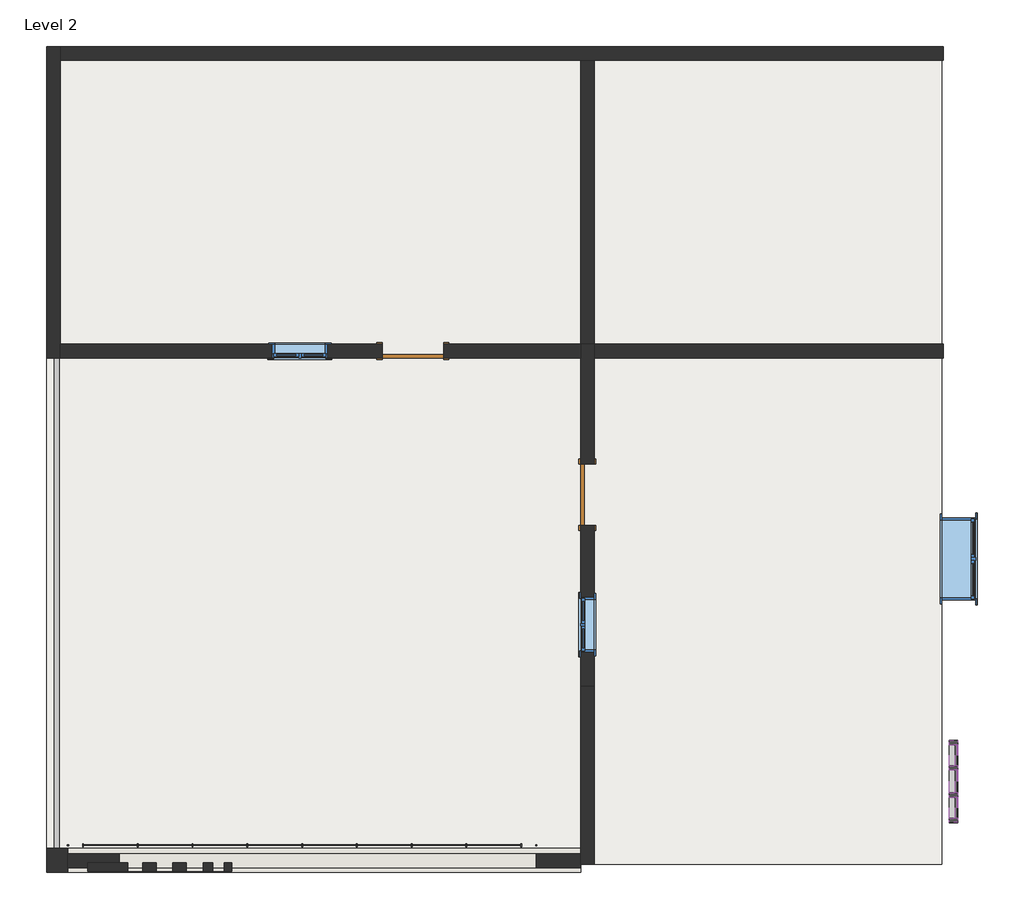
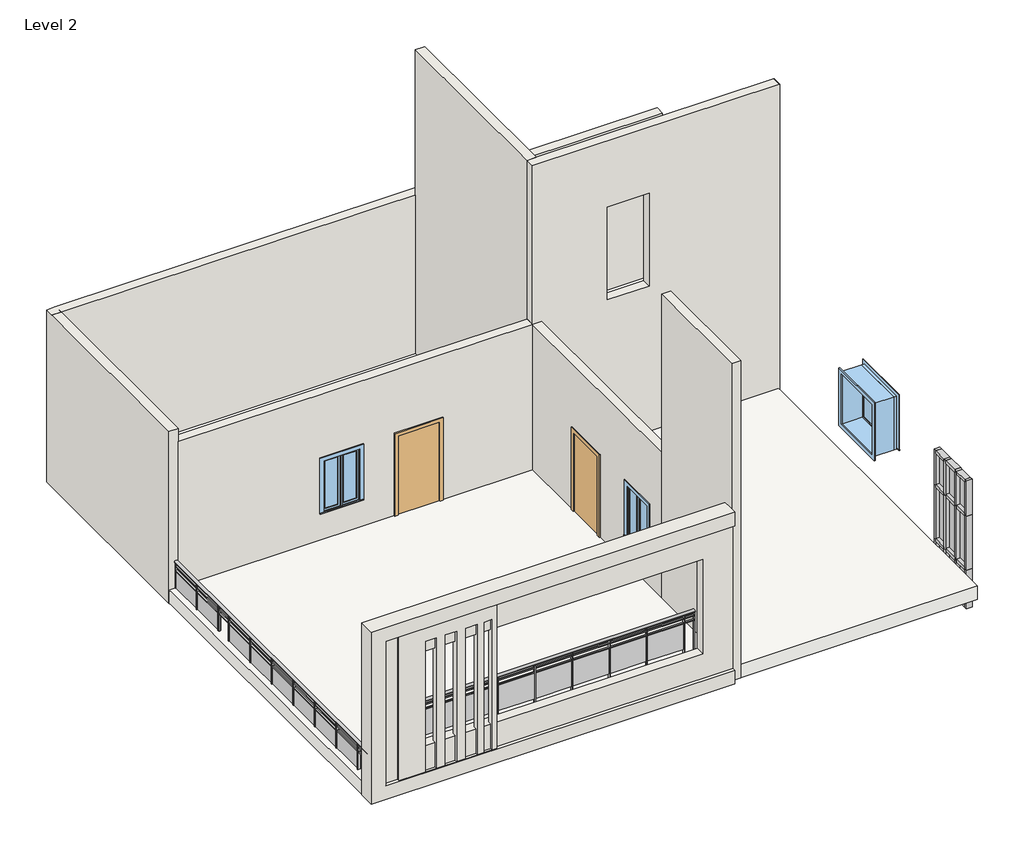
# One storey: 24 members, 10 walls, 9 plates, 3 windows, 2 doors, 2 railings, 1 roof.
"""IFC4 building model written with IfcOpenShell, lengths in millimetres."""

from ifc_helpers import new_model, si_unit, point, frame, origin, place, context, project, spatial, polyline, ellipse_curve, trimmed, outline, extrude, faceted_brep, transform, mapped, element, save
from ifc_brep_helpers import plane_surface, extruded_surface, advanced_brep
from components import door_54dd4da4, member_ff1b7d8f, member_5ad95953, member_5aeb4b7d, member_9850ab14, member_6e431393, member_26863f11, member_a1da5be3, member_58a4a87b, member_71eb4692, member_8b3492ed, system_panel_glazed_1557c927, system_panel_glazed_603fb926, system_panel_glazed_6328bcbd, system_panel_glazed_ea4b41a2, system_panel_glazed_510f06c2, system_panel_glazed_bd2ad356, walls_2_walls_2_aacfb59a, walls_3_walls_3_aaa7465c, window_bb17773d, window_25ed8443

model = new_model("IFC4")

# Units and contexts
model_context = context("Model", 3, world=origin())
ifc_project = project(units=[si_unit("LENGTHUNIT", "METRE", prefix="MILLI")], contexts=[model_context])

# Site, building, storey
site = spatial("IfcSite", under=ifc_project)
building = spatial("IfcBuilding", under=site)
storey = spatial("IfcBuildingStorey", under=building, Name="Level 2", Elevation=3657.6)

# Doors
placement = place(None, origin())
door_shape = door_54dd4da4(model_context)
element("IfcDoor", 1, ObjectType="Single-Flush : 36\" x 84\"", at=placement, inside=storey, context=model_context, shape_type="MappedRepresentation", body=[
    mapped(door_shape, transform((-6414.8745124, 6836.8609482, 3657.6), x_axis=(-1.0, 0.0, 0.0), y_axis=(0.0, -1.0, 0.0), z_axis=(0.0, 0.0, 1.0))),
])
element("IfcDoor", 2, ObjectType="Single-Flush : 36\" x 84\"", at=placement, inside=storey, context=model_context, shape_type="MappedRepresentation", body=[
    mapped(door_shape, transform((-3824.0745124, 4703.2609482, 3657.6), x_axis=(0.0, 1.0, 0.0), y_axis=(-1.0, 0.0, 0.0), z_axis=(0.0, 0.0, 1.0))),
])

# Members
member_shape = member_ff1b7d8f(model_context)
element("IfcMember", 3, ObjectType="Rectangular Mullion : 2.5\" x 5\" rectangular", at=placement, inside=storey, context=model_context, shape_type="MappedRepresentation", body=[
    mapped(member_shape, transform((1611.5254876, 617.0832725, 3022.9019988), x_axis=(0.0, 0.0, -1.0), y_axis=(-1.0, 0.0, 0.0), z_axis=(0.0, 1.0, 0.0))),
])
member_2_shape = member_5ad95953(model_context)
element("IfcMember", 4, ObjectType="Rectangular Mullion : 2.5\" x 5\" rectangular", at=placement, inside=storey, context=model_context, shape_type="MappedRepresentation", body=[
    mapped(member_2_shape, transform((1611.5254876, 210.6832725, 3022.9019988), x_axis=(0.0, 0.0, -1.0), y_axis=(-1.0, 0.0, 0.0), z_axis=(0.0, 1.0, 0.0))),
])
element("IfcMember", 5, ObjectType="Rectangular Mullion : 2.5\" x 5\" rectangular", at=placement, inside=storey, context=model_context, shape_type="MappedRepresentation", body=[
    mapped(member_2_shape, transform((1611.5254876, 991.7332725, 3022.9019988), x_axis=(0.0, 0.0, -1.0), y_axis=(-1.0, 0.0, 0.0), z_axis=(0.0, 1.0, 0.0))),
])
member_3_shape = member_5aeb4b7d(model_context)
element("IfcMember", 6, ObjectType="Rectangular Mullion : 2.5\" x 5\" rectangular", at=placement, inside=storey, context=model_context, shape_type="MappedRepresentation", body=[
    mapped(member_3_shape, transform((1611.5254876, 274.1832725, 3911.9019988), x_axis=(0.0, 0.0, 1.0), y_axis=(-1.0, 0.0, 0.0), z_axis=(0.0, -1.0, 0.0))),
])
element("IfcMember", 7, ObjectType="Rectangular Mullion : 2.5\" x 5\" rectangular", at=placement, inside=storey, context=model_context, shape_type="MappedRepresentation", body=[
    mapped(member_3_shape, transform((1611.5254876, 274.1832725, 5156.5019988), x_axis=(0.0, 0.0, 1.0), y_axis=(-1.0, 0.0, 0.0), z_axis=(0.0, -1.0, 0.0))),
])
member_4_shape = member_9850ab14(model_context)
element("IfcMember", 8, ObjectType="Rectangular Mullion : 2.5\" x 5\" rectangular", at=placement, inside=storey, context=model_context, shape_type="MappedRepresentation", body=[
    mapped(member_4_shape, transform((1611.5254876, -100.4667275, 3911.9019988), x_axis=(0.0, 0.0, 1.0), y_axis=(-1.0, 0.0, 0.0), z_axis=(0.0, -1.0, 0.0))),
])
element("IfcMember", 9, ObjectType="Rectangular Mullion : 2.5\" x 5\" rectangular", at=placement, inside=storey, context=model_context, shape_type="MappedRepresentation", body=[
    mapped(member_4_shape, transform((1611.5254876, 680.5832725, 3911.9019988), x_axis=(0.0, 0.0, 1.0), y_axis=(-1.0, 0.0, 0.0), z_axis=(0.0, -1.0, 0.0))),
])
element("IfcMember", 10, ObjectType="Rectangular Mullion : 2.5\" x 5\" rectangular", at=placement, inside=storey, context=model_context, shape_type="MappedRepresentation", body=[
    mapped(member_4_shape, transform((1611.5254876, -100.4667275, 5156.5019988), x_axis=(0.0, 0.0, 1.0), y_axis=(-1.0, 0.0, 0.0), z_axis=(0.0, -1.0, 0.0))),
])
element("IfcMember", 11, ObjectType="Rectangular Mullion : 2.5\" x 5\" rectangular", at=placement, inside=storey, context=model_context, shape_type="MappedRepresentation", body=[
    mapped(member_4_shape, transform((1611.5254876, 680.5832725, 5156.5019988), x_axis=(0.0, 0.0, 1.0), y_axis=(-1.0, 0.0, 0.0), z_axis=(0.0, -1.0, 0.0))),
])
element("IfcMember", 12, ObjectType="Rectangular Mullion : 2.5\" x 5\" rectangular", at=placement, inside=storey, context=model_context, shape_type="MappedRepresentation", body=[
    mapped(member_2_shape, transform((1611.5254876, 680.5832725, 5969.3019988), x_axis=(0.0, 0.0, 1.0), y_axis=(-1.0, 0.0, 0.0), z_axis=(0.0, -1.0, 0.0))),
])
element("IfcMember", 13, ObjectType="Rectangular Mullion : 2.5\" x 5\" rectangular", at=placement, inside=storey, context=model_context, shape_type="MappedRepresentation", body=[
    mapped(member_2_shape, transform((1611.5254876, -100.4667275, 5969.3019988), x_axis=(0.0, 0.0, 1.0), y_axis=(-1.0, 0.0, 0.0), z_axis=(0.0, -1.0, 0.0))),
])
element("IfcMember", 14, ObjectType="Rectangular Mullion : 2.5\" x 5\" rectangular", at=placement, inside=storey, context=model_context, shape_type="MappedRepresentation", body=[
    mapped(member_shape, transform((1611.5254876, 274.1832725, 5969.3019988), x_axis=(0.0, 0.0, 1.0), y_axis=(-1.0, 0.0, 0.0), z_axis=(0.0, -1.0, 0.0))),
])
member_5_shape = member_6e431393(model_context)
element("IfcMember", 15, ObjectType="Rectangular Mullion : 2.5\" x 5\" rectangular", at=placement, inside=storey, context=model_context, shape_type="MappedRepresentation", body=[
    mapped(member_5_shape, transform((1611.5254876, 648.8332725, 3022.9019988), x_axis=(0.0, -1.0, 0.0), y_axis=(-1.0, 0.0, 0.0), z_axis=(0.0, 0.0, -1.0))),
])
element("IfcMember", 16, ObjectType="Rectangular Mullion : 2.5\" x 5\" rectangular", at=placement, inside=storey, context=model_context, shape_type="MappedRepresentation", body=[
    mapped(member_5_shape, transform((1611.5254876, 242.4332725, 3022.9019988), x_axis=(0.0, -1.0, 0.0), y_axis=(-1.0, 0.0, 0.0), z_axis=(0.0, 0.0, -1.0))),
])
member_6_shape = member_26863f11(model_context)
element("IfcMember", 17, ObjectType="Rectangular Mullion : 2.5\" x 5\" rectangular", at=placement, inside=storey, context=model_context, shape_type="MappedRepresentation", body=[
    mapped(member_6_shape, transform((1611.5254876, -163.9667275, 3022.9019988), x_axis=(0.0, -1.0, 0.0), y_axis=(-1.0, 0.0, 0.0), z_axis=(0.0, 0.0, -1.0))),
])
element("IfcMember", 18, ObjectType="Rectangular Mullion : 2.5\" x 5\" rectangular", at=placement, inside=storey, context=model_context, shape_type="MappedRepresentation", body=[
    mapped(member_6_shape, transform((1611.5254876, 1055.2332725, 3911.9019988), x_axis=(0.0, 1.0, 0.0), y_axis=(-1.0, 0.0, 0.0), z_axis=(0.0, 0.0, 1.0))),
])
member_7_shape = member_a1da5be3(model_context)
element("IfcMember", 19, ObjectType="Rectangular Mullion : 2.5\" x 5\" rectangular", at=placement, inside=storey, context=model_context, shape_type="MappedRepresentation", body=[
    mapped(member_7_shape, transform((1611.5254876, 648.8332725, 3911.9019988), x_axis=(0.0, -1.0, 0.0), y_axis=(-1.0, 0.0, 0.0), z_axis=(0.0, 0.0, -1.0))),
])
element("IfcMember", 20, ObjectType="Rectangular Mullion : 2.5\" x 5\" rectangular", at=placement, inside=storey, context=model_context, shape_type="MappedRepresentation", body=[
    mapped(member_7_shape, transform((1611.5254876, 242.4332725, 3911.9019988), x_axis=(0.0, -1.0, 0.0), y_axis=(-1.0, 0.0, 0.0), z_axis=(0.0, 0.0, -1.0))),
])
member_8_shape = member_58a4a87b(model_context)
element("IfcMember", 21, ObjectType="Rectangular Mullion : 2.5\" x 5\" rectangular", at=placement, inside=storey, context=model_context, shape_type="MappedRepresentation", body=[
    mapped(member_8_shape, transform((1611.5254876, 648.8332725, 5156.5019988), x_axis=(0.0, -1.0, 0.0), y_axis=(-1.0, 0.0, 0.0), z_axis=(0.0, 0.0, -1.0))),
])
element("IfcMember", 22, ObjectType="Rectangular Mullion : 2.5\" x 5\" rectangular", at=placement, inside=storey, context=model_context, shape_type="MappedRepresentation", body=[
    mapped(member_8_shape, transform((1611.5254876, 242.4332725, 5156.5019988), x_axis=(0.0, -1.0, 0.0), y_axis=(-1.0, 0.0, 0.0), z_axis=(0.0, 0.0, -1.0))),
])
member_9_shape = member_71eb4692(model_context)
element("IfcMember", 23, ObjectType="Rectangular Mullion : 2.5\" x 5\" rectangular", at=placement, inside=storey, context=model_context, shape_type="MappedRepresentation", body=[
    mapped(member_9_shape, transform((1611.5254876, -163.9667275, 3911.9019988), x_axis=(0.0, -1.0, 0.0), y_axis=(-1.0, 0.0, 0.0), z_axis=(0.0, 0.0, -1.0))),
])
member_10_shape = member_8b3492ed(model_context)
element("IfcMember", 24, ObjectType="Rectangular Mullion : 2.5\" x 5\" rectangular", at=placement, inside=storey, context=model_context, shape_type="MappedRepresentation", body=[
    mapped(member_10_shape, transform((1611.5254876, -163.9667275, 5156.5019988), x_axis=(0.0, -1.0, 0.0), y_axis=(-1.0, 0.0, 0.0), z_axis=(0.0, 0.0, -1.0))),
])
element("IfcMember", 25, ObjectType="Rectangular Mullion : 2.5\" x 5\" rectangular", at=placement, inside=storey, context=model_context, shape_type="MappedRepresentation", body=[
    mapped(member_9_shape, transform((1611.5254876, 1055.2332725, 5156.5019988), x_axis=(0.0, 1.0, 0.0), y_axis=(-1.0, 0.0, 0.0), z_axis=(0.0, 0.0, 1.0))),
])
element("IfcMember", 26, ObjectType="Rectangular Mullion : 2.5\" x 5\" rectangular", at=placement, inside=storey, context=model_context, shape_type="MappedRepresentation", body=[
    mapped(member_10_shape, transform((1611.5254876, 1055.2332725, 5969.3019988), x_axis=(0.0, 1.0, 0.0), y_axis=(-1.0, 0.0, 0.0), z_axis=(0.0, 0.0, 1.0))),
])

# Plates
system_panel_glazed_shape = system_panel_glazed_1557c927(model_context)
element("IfcPlate", 27, ObjectType="System Panel : Glazed", at=placement, inside=storey, context=model_context, shape_type="MappedRepresentation", body=[
    mapped(system_panel_glazed_shape, transform((1611.5254876, 836.1582725, 3086.4019988), x_axis=(0.0, -1.0, 0.0), y_axis=(1.0, 0.0, 0.0), z_axis=(0.0, 0.0, 1.0))),
])
element("IfcPlate", 28, ObjectType="System Panel : Glazed", at=placement, inside=storey, context=model_context, shape_type="MappedRepresentation", body=[
    mapped(system_panel_glazed_shape, transform((1611.5254876, 55.1082725, 3086.4019988), x_axis=(0.0, -1.0, 0.0), y_axis=(1.0, 0.0, 0.0), z_axis=(0.0, 0.0, 1.0))),
])
system_panel_glazed_2_shape = system_panel_glazed_603fb926(model_context)
element("IfcPlate", 29, ObjectType="System Panel : Glazed", at=placement, inside=storey, context=model_context, shape_type="MappedRepresentation", body=[
    mapped(system_panel_glazed_2_shape, transform((1611.5254876, 445.6332725, 3086.4019988), x_axis=(0.0, -1.0, 0.0), y_axis=(1.0, 0.0, 0.0), z_axis=(0.0, 0.0, 1.0))),
])
system_panel_glazed_3_shape = system_panel_glazed_6328bcbd(model_context)
element("IfcPlate", 30, ObjectType="System Panel : Glazed", at=placement, inside=storey, context=model_context, shape_type="MappedRepresentation", body=[
    mapped(system_panel_glazed_3_shape, transform((1611.5254876, 836.1582725, 5188.2519988), x_axis=(0.0, -1.0, 0.0), y_axis=(1.0, 0.0, 0.0), z_axis=(0.0, 0.0, 1.0))),
])
element("IfcPlate", 31, ObjectType="System Panel : Glazed", at=placement, inside=storey, context=model_context, shape_type="MappedRepresentation", body=[
    mapped(system_panel_glazed_3_shape, transform((1611.5254876, 55.1082725, 5188.2519988), x_axis=(0.0, -1.0, 0.0), y_axis=(1.0, 0.0, 0.0), z_axis=(0.0, 0.0, 1.0))),
])
system_panel_glazed_4_shape = system_panel_glazed_ea4b41a2(model_context)
element("IfcPlate", 32, ObjectType="System Panel : Glazed", at=placement, inside=storey, context=model_context, shape_type="MappedRepresentation", body=[
    mapped(system_panel_glazed_4_shape, transform((1611.5254876, 445.6332725, 5188.2519988), x_axis=(0.0, -1.0, 0.0), y_axis=(1.0, 0.0, 0.0), z_axis=(0.0, 0.0, 1.0))),
])
system_panel_glazed_5_shape = system_panel_glazed_510f06c2(model_context)
element("IfcPlate", 33, ObjectType="System Panel : Glazed", at=placement, inside=storey, context=model_context, shape_type="MappedRepresentation", body=[
    mapped(system_panel_glazed_5_shape, transform((1611.5254876, 836.1582725, 3943.6519988), x_axis=(0.0, -1.0, 0.0), y_axis=(1.0, 0.0, 0.0), z_axis=(0.0, 0.0, 1.0))),
])
element("IfcPlate", 34, ObjectType="System Panel : Glazed", at=placement, inside=storey, context=model_context, shape_type="MappedRepresentation", body=[
    mapped(system_panel_glazed_5_shape, transform((1611.5254876, 55.1082725, 3943.6519988), x_axis=(0.0, -1.0, 0.0), y_axis=(1.0, 0.0, 0.0), z_axis=(0.0, 0.0, 1.0))),
])
system_panel_glazed_6_shape = system_panel_glazed_bd2ad356(model_context)
element("IfcPlate", 35, ObjectType="System Panel : Glazed", at=placement, inside=storey, context=model_context, shape_type="MappedRepresentation", body=[
    mapped(system_panel_glazed_6_shape, transform((1611.5254876, 445.6332725, 3943.6519988), x_axis=(0.0, -1.0, 0.0), y_axis=(1.0, 0.0, 0.0), z_axis=(0.0, 0.0, 1.0))),
])

# Railings
element("IfcRailing", 36, ObjectType="Glass Panel - Bottom Fill", at=placement, inside=storey, context=model_context, shape_type="SolidModel", body=[
    advanced_brep(
    [(-11535.2764802, -464.1328007, 5334.0), (-11535.2764802, -540.3328007, 5334.0), (-4580.8162469, -464.1328007, 5334.0), (-4580.8162469, -540.3328007, 5334.0)],
    [
        (0, 1, ellipse_curve(frame((-11535.2764802, -502.2328007, 5334.0), z_axis=(-1.0, 0.0, 0.0), x_axis=(0.0, -1.0, 0.0)), 38.1, 28.575)),
        (1, 0, ellipse_curve(frame((-11535.2764802, -502.2328007, 5334.0), z_axis=(-1.0, 0.0, 0.0), x_axis=(0.0, -1.0, 0.0)), 38.1, 28.575)),
        (2, 3, ellipse_curve(frame((-4580.8162469, -502.2328007, 5334.0), z_axis=(1.0, 0.0, 0.0), x_axis=(0.0, -1.0, 0.0)), 38.1, 28.575)),
        (3, 2, ellipse_curve(frame((-4580.8162469, -502.2328007, 5334.0), z_axis=(1.0, 0.0, 0.0), x_axis=(0.0, -1.0, 0.0)), 38.1, 28.575)),
        (0, 2),
        (3, 1),
    ],
    [
        plane_surface(frame((-11535.2764802, -502.2328007, 5334.0), z_axis=(-1.0, 0.0, 0.0), x_axis=(0.0, 1.0, 0.0))),
        plane_surface(frame((-4580.8162469, -502.2328007, 5334.0), z_axis=(1.0, 0.0, 0.0), x_axis=(0.0, 1.0, 0.0))),
        extruded_surface(trimmed(ellipse_curve(frame((-4580.8162469, -502.2328007, 5334.0), z_axis=(-1.0, 0.0, 0.0), x_axis=(0.0, -1.0, 0.0)), 38.1, 28.575), [point((-4580.8162469, -464.1328007, 5334.0))], [point((-4580.8162469, -540.3328007, 5334.0))], True, "CARTESIAN"), (-6954.4602333, 0.0, 0.0), 6954.4602333),
        extruded_surface(trimmed(ellipse_curve(frame((-4580.8162469, -502.2328007, 5334.0), z_axis=(-1.0, 0.0, 0.0), x_axis=(0.0, -1.0, 0.0)), 38.1, 28.575), [point((-4580.8162469, -540.3328007, 5334.0))], [point((-4580.8162469, -464.1328007, 5334.0))], True, "CARTESIAN"), (-6954.4602333, 0.0, 0.0), 6954.4602333),
    ],
    [
        (0, [[1, 2]]),
        (1, [[3, 4]]),
        (2, [[-1, 5, -4, 6]]),
        (3, [[-2, -6, -3, -5]]),
    ],
),
    extrude(outline(polyline([(-11535.2764802, -514.9328007), (-11535.2764802, -489.5328007), (-4580.8162469, -489.5328007), (-4580.8162469, -514.9328007), (-11535.2764802, -514.9328007)])), frame((0.0, 0.0, 5219.7), z_axis=(0.0, 0.0, 1.0), x_axis=(1.0, 0.0, 0.0)), (0.0, 0.0, 1.0), 25.4),
    extrude(outline(polyline([(-11535.2764802, -514.9328007), (-11535.2764802, -489.5328007), (-4580.8162469, -489.5328007), (-4580.8162469, -514.9328007), (-11535.2764802, -514.9328007)])), frame((0.0, 0.0, 5118.1), z_axis=(0.0, 0.0, 1.0), x_axis=(1.0, 0.0, 0.0)), (0.0, 0.0, 1.0), 25.4),
    extrude(outline(polyline([(-4813.1963636, -527.6328007), (-4813.1963636, -476.8328007), (-4800.4963636, -476.8328007), (-4800.4963636, -527.6328007), (-4813.1963636, -527.6328007)])), frame((0.0, 0.0, 4419.6), z_axis=(0.0, 0.0, 1.0), x_axis=(1.0, 0.0, 0.0)), (0.0, 0.0, 1.0), 885.6788223),
    extrude(outline(polyline([(-5619.6463636, -495.6976436), (-4806.8463636, -495.6976436), (-4806.8463636, -502.0476436), (-5619.6463636, -502.0476436), (-5619.6463636, -495.6976436)])), frame((0.0, 0.0, 4521.2), z_axis=(0.0, 0.0, 1.0), x_axis=(1.0, 0.0, 0.0)), (0.0, 0.0, 1.0), 596.9),
    extrude(outline(polyline([(-5625.9963636, -527.6328007), (-5625.9963636, -476.8328007), (-5613.2963636, -476.8328007), (-5613.2963636, -527.6328007), (-5625.9963636, -527.6328007)])), frame((0.0, 0.0, 4419.6), z_axis=(0.0, 0.0, 1.0), x_axis=(1.0, 0.0, 0.0)), (0.0, 0.0, 1.0), 885.6788223),
    extrude(outline(polyline([(-6432.4463636, -495.6976436), (-5619.6463636, -495.6976436), (-5619.6463636, -502.0476436), (-6432.4463636, -502.0476436), (-6432.4463636, -495.6976436)])), frame((0.0, 0.0, 4521.2), z_axis=(0.0, 0.0, 1.0), x_axis=(1.0, 0.0, 0.0)), (0.0, 0.0, 1.0), 596.9),
    extrude(outline(polyline([(-6438.7963636, -527.6328007), (-6438.7963636, -476.8328007), (-6426.0963636, -476.8328007), (-6426.0963636, -527.6328007), (-6438.7963636, -527.6328007)])), frame((0.0, 0.0, 4419.6), z_axis=(0.0, 0.0, 1.0), x_axis=(1.0, 0.0, 0.0)), (0.0, 0.0, 1.0), 885.6788223),
    extrude(outline(polyline([(-7245.2463636, -495.6976436), (-6432.4463636, -495.6976436), (-6432.4463636, -502.0476436), (-7245.2463636, -502.0476436), (-7245.2463636, -495.6976436)])), frame((0.0, 0.0, 4521.2), z_axis=(0.0, 0.0, 1.0), x_axis=(1.0, 0.0, 0.0)), (0.0, 0.0, 1.0), 596.9),
    extrude(outline(polyline([(-7251.5963636, -527.6328007), (-7251.5963636, -476.8328007), (-7238.8963636, -476.8328007), (-7238.8963636, -527.6328007), (-7251.5963636, -527.6328007)])), frame((0.0, 0.0, 4419.6), z_axis=(0.0, 0.0, 1.0), x_axis=(1.0, 0.0, 0.0)), (0.0, 0.0, 1.0), 885.6788223),
    extrude(outline(polyline([(-8058.0463636, -495.6976436), (-7245.2463636, -495.6976436), (-7245.2463636, -502.0476436), (-8058.0463636, -502.0476436), (-8058.0463636, -495.6976436)])), frame((0.0, 0.0, 4521.2), z_axis=(0.0, 0.0, 1.0), x_axis=(1.0, 0.0, 0.0)), (0.0, 0.0, 1.0), 596.9),
    extrude(outline(polyline([(-8064.3963636, -527.6328007), (-8064.3963636, -476.8328007), (-8051.6963636, -476.8328007), (-8051.6963636, -527.6328007), (-8064.3963636, -527.6328007)])), frame((0.0, 0.0, 4419.6), z_axis=(0.0, 0.0, 1.0), x_axis=(1.0, 0.0, 0.0)), (0.0, 0.0, 1.0), 885.6788223),
    extrude(outline(polyline([(-8870.8463636, -495.6976436), (-8058.0463636, -495.6976436), (-8058.0463636, -502.0476436), (-8870.8463636, -502.0476436), (-8870.8463636, -495.6976436)])), frame((0.0, 0.0, 4521.2), z_axis=(0.0, 0.0, 1.0), x_axis=(1.0, 0.0, 0.0)), (0.0, 0.0, 1.0), 596.9),
    extrude(outline(polyline([(-8877.1963636, -527.6328007), (-8877.1963636, -476.8328007), (-8864.4963636, -476.8328007), (-8864.4963636, -527.6328007), (-8877.1963636, -527.6328007)])), frame((0.0, 0.0, 4419.6), z_axis=(0.0, 0.0, 1.0), x_axis=(1.0, 0.0, 0.0)), (0.0, 0.0, 1.0), 885.6788223),
    extrude(outline(polyline([(-9683.6463636, -495.6976436), (-8870.8463636, -495.6976436), (-8870.8463636, -502.0476436), (-9683.6463636, -502.0476436), (-9683.6463636, -495.6976436)])), frame((0.0, 0.0, 4521.2), z_axis=(0.0, 0.0, 1.0), x_axis=(1.0, 0.0, 0.0)), (0.0, 0.0, 1.0), 596.9),
    extrude(outline(polyline([(-9689.9963636, -527.6328007), (-9689.9963636, -476.8328007), (-9677.2963636, -476.8328007), (-9677.2963636, -527.6328007), (-9689.9963636, -527.6328007)])), frame((0.0, 0.0, 4419.6), z_axis=(0.0, 0.0, 1.0), x_axis=(1.0, 0.0, 0.0)), (0.0, 0.0, 1.0), 885.6788223),
    extrude(outline(polyline([(-10496.4463636, -495.6976436), (-9683.6463636, -495.6976436), (-9683.6463636, -502.0476436), (-10496.4463636, -502.0476436), (-10496.4463636, -495.6976436)])), frame((0.0, 0.0, 4521.2), z_axis=(0.0, 0.0, 1.0), x_axis=(1.0, 0.0, 0.0)), (0.0, 0.0, 1.0), 596.9),
    extrude(outline(polyline([(-10502.7963636, -527.6328007), (-10502.7963636, -476.8328007), (-10490.0963636, -476.8328007), (-10490.0963636, -527.6328007), (-10502.7963636, -527.6328007)])), frame((0.0, 0.0, 4419.6), z_axis=(0.0, 0.0, 1.0), x_axis=(1.0, 0.0, 0.0)), (0.0, 0.0, 1.0), 885.6788223),
    extrude(outline(polyline([(-11309.2463636, -495.6976436), (-10496.4463636, -495.6976436), (-10496.4463636, -502.0476436), (-11309.2463636, -502.0476436), (-11309.2463636, -495.6976436)])), frame((0.0, 0.0, 4521.2), z_axis=(0.0, 0.0, 1.0), x_axis=(1.0, 0.0, 0.0)), (0.0, 0.0, 1.0), 596.9),
    extrude(outline(polyline([(-11315.5963636, -527.6328007), (-11315.5963636, -476.8328007), (-11302.8963636, -476.8328007), (-11302.8963636, -527.6328007), (-11315.5963636, -527.6328007)])), frame((0.0, 0.0, 4419.6), z_axis=(0.0, 0.0, 1.0), x_axis=(1.0, 0.0, 0.0)), (0.0, 0.0, 1.0), 885.6788223),
    extrude(outline(polyline([(-4593.5162469, -511.7578007), (-4593.5162469, -492.7078007), (-4574.4662469, -492.7078007), (-4574.4662469, -511.7578007), (-4593.5162469, -511.7578007)])), frame((0.0, 0.0, 4419.6), z_axis=(0.0, 0.0, 1.0), x_axis=(1.0, 0.0, 0.0)), (0.0, 0.0, 1.0), 885.6788223),
    extrude(outline(polyline([(-11541.6264802, -511.7578007), (-11541.6264802, -492.7078007), (-11522.5764802, -492.7078007), (-11522.5764802, -511.7578007), (-11541.6264802, -511.7578007)])), frame((0.0, 0.0, 4419.6), z_axis=(0.0, 0.0, 1.0), x_axis=(1.0, 0.0, 0.0)), (0.0, 0.0, 1.0), 885.6788223),
])
element("IfcRailing", 37, ObjectType="Glass Panel - Bottom Fill", at=placement, inside=storey, context=model_context, shape_type="SolidModel", body=[
    advanced_brep(
    [(-11736.1745124, -545.7345899, 4572.0), (-11659.9745124, -545.7345899, 4572.0), (-11736.1745124, 6735.2609482, 4572.0), (-11659.9745124, 6735.2609482, 4572.0)],
    [
        (0, 1, ellipse_curve(frame((-11698.0745124, -545.7345899, 4572.0), z_axis=(0.0, -1.0, 0.0), x_axis=(1.0, 0.0, 0.0)), 38.1, 28.575)),
        (1, 0, ellipse_curve(frame((-11698.0745124, -545.7345899, 4572.0), z_axis=(0.0, -1.0, 0.0), x_axis=(1.0, 0.0, 0.0)), 38.1, 28.575)),
        (2, 3, ellipse_curve(frame((-11698.0745124, 6735.2609482, 4572.0), z_axis=(0.0, 1.0, 0.0), x_axis=(1.0, 0.0, 0.0)), 38.1, 28.575)),
        (3, 2, ellipse_curve(frame((-11698.0745124, 6735.2609482, 4572.0), z_axis=(0.0, 1.0, 0.0), x_axis=(1.0, 0.0, 0.0)), 38.1, 28.575)),
        (0, 2),
        (3, 1),
    ],
    [
        plane_surface(frame((-11698.0745124, -545.7345899, 4572.0), z_axis=(0.0, -1.0, 0.0), x_axis=(0.0, 0.0, 1.0))),
        plane_surface(frame((-11698.0745124, 6735.2609482, 4572.0), z_axis=(0.0, 1.0, 0.0), x_axis=(0.0, 0.0, 1.0))),
        extruded_surface(trimmed(ellipse_curve(frame((-11698.0745124, 6735.2609482, 4572.0), z_axis=(0.0, -1.0, 0.0), x_axis=(1.0, 0.0, 0.0)), 38.1, 28.575), [point((-11736.1745124, 6735.2609482, 4572.0))], [point((-11659.9745124, 6735.2609482, 4572.0))], True, "CARTESIAN"), (0.0, -7280.9955381, 0.0), 7280.9955381),
        extruded_surface(trimmed(ellipse_curve(frame((-11698.0745124, 6735.2609482, 4572.0), z_axis=(0.0, -1.0, 0.0), x_axis=(1.0, 0.0, 0.0)), 38.1, 28.575), [point((-11659.9745124, 6735.2609482, 4572.0))], [point((-11736.1745124, 6735.2609482, 4572.0))], True, "CARTESIAN"), (0.0, -7280.9955381, 0.0), 7280.9955381),
    ],
    [
        (0, [[1, 2]]),
        (1, [[3, 4]]),
        (2, [[-1, 5, -4, 6]]),
        (3, [[-2, -6, -3, -5]]),
    ],
),
    extrude(outline(polyline([(-11685.3745124, -545.7345899), (-11710.7745124, -545.7345899), (-11710.7745124, 6735.2609482), (-11685.3745124, 6735.2609482), (-11685.3745124, -545.7345899)])), frame((0.0, 0.0, 4457.7), z_axis=(0.0, 0.0, 1.0), x_axis=(1.0, 0.0, 0.0)), (0.0, 0.0, 1.0), 25.4),
    extrude(outline(polyline([(-11685.3745124, -545.7345899), (-11710.7745124, -545.7345899), (-11710.7745124, 6735.2609482), (-11685.3745124, 6735.2609482), (-11685.3745124, -545.7345899)])), frame((0.0, 0.0, 4356.1), z_axis=(0.0, 0.0, 1.0), x_axis=(1.0, 0.0, 0.0)), (0.0, 0.0, 1.0), 25.4),
    extrude(outline(polyline([(-11672.6745124, 6720.6131791), (-11723.4745124, 6720.6131791), (-11723.4745124, 6733.3131791), (-11672.6745124, 6733.3131791), (-11672.6745124, 6720.6131791)])), frame((0.0, 0.0, 3657.6), z_axis=(0.0, 0.0, 1.0), x_axis=(1.0, 0.0, 0.0)), (0.0, 0.0, 1.0), 885.6788223),
    extrude(outline(polyline([(-11704.6096694, 5914.1631791), (-11704.6096694, 6726.9631791), (-11698.2596694, 6726.9631791), (-11698.2596694, 5914.1631791), (-11704.6096694, 5914.1631791)])), frame((0.0, 0.0, 3759.2), z_axis=(0.0, 0.0, 1.0), x_axis=(1.0, 0.0, 0.0)), (0.0, 0.0, 1.0), 596.9),
    extrude(outline(polyline([(-11672.6745124, 5907.8131791), (-11723.4745124, 5907.8131791), (-11723.4745124, 5920.5131791), (-11672.6745124, 5920.5131791), (-11672.6745124, 5907.8131791)])), frame((0.0, 0.0, 3657.6), z_axis=(0.0, 0.0, 1.0), x_axis=(1.0, 0.0, 0.0)), (0.0, 0.0, 1.0), 885.6788223),
    extrude(outline(polyline([(-11704.6096694, 5101.3631791), (-11704.6096694, 5914.1631791), (-11698.2596694, 5914.1631791), (-11698.2596694, 5101.3631791), (-11704.6096694, 5101.3631791)])), frame((0.0, 0.0, 3759.2), z_axis=(0.0, 0.0, 1.0), x_axis=(1.0, 0.0, 0.0)), (0.0, 0.0, 1.0), 596.9),
    extrude(outline(polyline([(-11672.6745124, 5095.0131791), (-11723.4745124, 5095.0131791), (-11723.4745124, 5107.7131791), (-11672.6745124, 5107.7131791), (-11672.6745124, 5095.0131791)])), frame((0.0, 0.0, 3657.6), z_axis=(0.0, 0.0, 1.0), x_axis=(1.0, 0.0, 0.0)), (0.0, 0.0, 1.0), 885.6788223),
    extrude(outline(polyline([(-11672.6745124, 4705.7154101), (-11723.4745124, 4705.7154101), (-11723.4745124, 4718.4154101), (-11672.6745124, 4718.4154101), (-11672.6745124, 4705.7154101)])), frame((0.0, 0.0, 3657.6), z_axis=(0.0, 0.0, 1.0), x_axis=(1.0, 0.0, 0.0)), (0.0, 0.0, 1.0), 885.6788223),
    extrude(outline(polyline([(-11704.6096694, 3899.2654101), (-11704.6096694, 4712.0654101), (-11698.2596694, 4712.0654101), (-11698.2596694, 3899.2654101), (-11704.6096694, 3899.2654101)])), frame((0.0, 0.0, 3759.2), z_axis=(0.0, 0.0, 1.0), x_axis=(1.0, 0.0, 0.0)), (0.0, 0.0, 1.0), 596.9),
    extrude(outline(polyline([(-11672.6745124, 3892.9154101), (-11723.4745124, 3892.9154101), (-11723.4745124, 3905.6154101), (-11672.6745124, 3905.6154101), (-11672.6745124, 3892.9154101)])), frame((0.0, 0.0, 3657.6), z_axis=(0.0, 0.0, 1.0), x_axis=(1.0, 0.0, 0.0)), (0.0, 0.0, 1.0), 885.6788223),
    extrude(outline(polyline([(-11704.6096694, 3086.4654101), (-11704.6096694, 3899.2654101), (-11698.2596694, 3899.2654101), (-11698.2596694, 3086.4654101), (-11704.6096694, 3086.4654101)])), frame((0.0, 0.0, 3759.2), z_axis=(0.0, 0.0, 1.0), x_axis=(1.0, 0.0, 0.0)), (0.0, 0.0, 1.0), 596.9),
    extrude(outline(polyline([(-11672.6745124, 3080.1154101), (-11723.4745124, 3080.1154101), (-11723.4745124, 3092.8154101), (-11672.6745124, 3092.8154101), (-11672.6745124, 3080.1154101)])), frame((0.0, 0.0, 3657.6), z_axis=(0.0, 0.0, 1.0), x_axis=(1.0, 0.0, 0.0)), (0.0, 0.0, 1.0), 885.6788223),
    extrude(outline(polyline([(-11704.6096694, 2273.6654101), (-11704.6096694, 3086.4654101), (-11698.2596694, 3086.4654101), (-11698.2596694, 2273.6654101), (-11704.6096694, 2273.6654101)])), frame((0.0, 0.0, 3759.2), z_axis=(0.0, 0.0, 1.0), x_axis=(1.0, 0.0, 0.0)), (0.0, 0.0, 1.0), 596.9),
    extrude(outline(polyline([(-11672.6745124, 2267.3154101), (-11723.4745124, 2267.3154101), (-11723.4745124, 2280.0154101), (-11672.6745124, 2280.0154101), (-11672.6745124, 2267.3154101)])), frame((0.0, 0.0, 3657.6), z_axis=(0.0, 0.0, 1.0), x_axis=(1.0, 0.0, 0.0)), (0.0, 0.0, 1.0), 885.6788223),
    extrude(outline(polyline([(-11704.6096694, 1460.8654101), (-11704.6096694, 2273.6654101), (-11698.2596694, 2273.6654101), (-11698.2596694, 1460.8654101), (-11704.6096694, 1460.8654101)])), frame((0.0, 0.0, 3759.2), z_axis=(0.0, 0.0, 1.0), x_axis=(1.0, 0.0, 0.0)), (0.0, 0.0, 1.0), 596.9),
    extrude(outline(polyline([(-11672.6745124, 1454.5154101), (-11723.4745124, 1454.5154101), (-11723.4745124, 1467.2154101), (-11672.6745124, 1467.2154101), (-11672.6745124, 1454.5154101)])), frame((0.0, 0.0, 3657.6), z_axis=(0.0, 0.0, 1.0), x_axis=(1.0, 0.0, 0.0)), (0.0, 0.0, 1.0), 885.6788223),
    extrude(outline(polyline([(-11704.6096694, 648.0654101), (-11704.6096694, 1460.8654101), (-11698.2596694, 1460.8654101), (-11698.2596694, 648.0654101), (-11704.6096694, 648.0654101)])), frame((0.0, 0.0, 3759.2), z_axis=(0.0, 0.0, 1.0), x_axis=(1.0, 0.0, 0.0)), (0.0, 0.0, 1.0), 596.9),
    extrude(outline(polyline([(-11672.6745124, 641.7154101), (-11723.4745124, 641.7154101), (-11723.4745124, 654.4154101), (-11672.6745124, 654.4154101), (-11672.6745124, 641.7154101)])), frame((0.0, 0.0, 3657.6), z_axis=(0.0, 0.0, 1.0), x_axis=(1.0, 0.0, 0.0)), (0.0, 0.0, 1.0), 885.6788223),
    extrude(outline(polyline([(-11704.6096694, -164.7345899), (-11704.6096694, 648.0654101), (-11698.2596694, 648.0654101), (-11698.2596694, -164.7345899), (-11704.6096694, -164.7345899)])), frame((0.0, 0.0, 3759.2), z_axis=(0.0, 0.0, 1.0), x_axis=(1.0, 0.0, 0.0)), (0.0, 0.0, 1.0), 596.9),
    extrude(outline(polyline([(-11672.6745124, -171.0845899), (-11723.4745124, -171.0845899), (-11723.4745124, -158.3845899), (-11672.6745124, -158.3845899), (-11672.6745124, -171.0845899)])), frame((0.0, 0.0, 3657.6), z_axis=(0.0, 0.0, 1.0), x_axis=(1.0, 0.0, 0.0)), (0.0, 0.0, 1.0), 885.6788223),
    extrude(outline(polyline([(-11688.5495124, 5083.5404101), (-11707.5995124, 5083.5404101), (-11707.5995124, 5102.5904101), (-11688.5495124, 5102.5904101), (-11688.5495124, 5083.5404101)])), frame((0.0, 0.0, 3657.6), z_axis=(0.0, 0.0, 1.0), x_axis=(1.0, 0.0, 0.0)), (0.0, 0.0, 1.0), 885.6788223),
    extrude(outline(polyline([(-11688.5495124, 6722.5609482), (-11707.5995124, 6722.5609482), (-11707.5995124, 6741.6109482), (-11688.5495124, 6741.6109482), (-11688.5495124, 6722.5609482)])), frame((0.0, 0.0, 3657.6), z_axis=(0.0, 0.0, 1.0), x_axis=(1.0, 0.0, 0.0)), (0.0, 0.0, 1.0), 885.6788223),
    extrude(outline(polyline([(-11688.5495124, -552.0845899), (-11707.5995124, -552.0845899), (-11707.5995124, -533.0345899), (-11688.5495124, -533.0345899), (-11688.5495124, -552.0845899)])), frame((0.0, 0.0, 3657.6), z_axis=(0.0, 0.0, 1.0), x_axis=(1.0, 0.0, 0.0)), (0.0, 0.0, 1.0), 885.6788223),
])

# Roof
element("IfcRoof", 38, ObjectType="Generic - 12\"", at=placement, inside=storey, context=model_context, shape_type="SweptSolid", body=[
    extrude(outline(polyline([(-11847.2995124, 11192.9609482), (1433.7254876, 11192.9609482), (1433.7254876, -783.1390518), (-11847.2995124, -783.1390518), (-11847.2995124, 11192.9609482)])), frame((0.0, 0.0, 3657.6), z_axis=(0.0, 0.0, 1.0), x_axis=(1.0, 0.0, 0.0)), (0.0, 0.0, 1.0), 304.8),
])

# Walls
element("IfcWall", 39, ObjectType="Generic - 5\"", at=placement, inside=storey, context=model_context, shape_type="SweptSolid", body=[
    extrude(outline(polyline([(3657.6, -11237.6995124), (3657.6, -9104.0995124), (7315.2, -9104.0995124), (7315.2, -11237.6995124), (3657.6, -11237.6995124)]), holes=[polyline([(6979.2767543, -10420.0050248), (3973.3839769, -10420.0050248), (3973.3839769, -10648.4418591), (6979.2767543, -10648.4418591), (6979.2767543, -10420.0050248)]), polyline([(6979.2767543, -9525.0088095), (3973.3839769, -9525.0088095), (3973.3839769, -9779.8810993), (6979.2767543, -9779.8810993), (6979.2767543, -9525.0088095)]), polyline([(6979.2767543, -9980.1378985), (3973.3839769, -9980.1378985), (3973.3839769, -10225.9076065), (6979.2767543, -10225.9076065), (6979.2767543, -9980.1378985)]), polyline([(6979.2767543, -9210.2339379), (3973.3839769, -9210.2339379), (3973.3839769, -9381.2752463), (6979.2767543, -9381.2752463), (6979.2767543, -9210.2339379)])]), frame((0.0, -884.7783837, 0.0), z_axis=(0.0, 1.0, 0.0), x_axis=(0.0, 0.0, 1.0)), (0.0, 0.0, 1.0), 127.0),
])
element("IfcWall", 40, ObjectType="Generic - 8\"", at=placement, inside=storey, context=model_context, shape_type="Brep", body=[
    faceted_brep([(-11850.4745124, 11358.0609482, 7620.0), (-11850.4745124, 11358.0609482, 3657.6), (-11850.4745124, 6735.2609482, 3657.6), (-11850.4745124, 6735.2609482, 7620.0), (-11850.4745124, 11154.8609482, 7620.0), (-11647.2745124, 11358.0609482, 3657.6), (-11647.2745124, 11358.0609482, 7315.2), (-11647.2745124, 11358.0609482, 7620.0), (-11647.2745124, 11154.8609482, 7620.0), (-11647.2745124, 6735.2609482, 7620.0), (-11647.2745124, 6735.2609482, 7315.2), (-11647.2745124, 6735.2609482, 3657.6), (-11647.2745124, 6938.4609482, 3657.6), (-11647.2745124, 11154.8609482, 3657.6)], [[[0, 1, 2, 3, 4]], [[5, 6, 7, 8, 9, 10, 11, 12, 13]], [[2, 1, 5, 13, 12, 11]], [[0, 4, 3, 9, 8, 7]], [[0, 7, 6, 5, 1]], [[2, 11, 10, 9, 3]]]),
])
element("IfcWall", 41, ObjectType="Generic - 8\"", at=placement, inside=storey, context=model_context, shape_type="Brep", body=[
    faceted_brep([(-3722.4745124, 5160.4609482, 5791.2), (-3722.4745124, 5160.4609482, 3657.6), (-3722.4745124, 6735.2609482, 3657.6), (-3722.4745124, 6938.4609482, 3657.6), (-3722.4745124, 6938.4609482, 7315.2), (-3722.4745124, 6735.2609482, 7315.2), (-3722.4745124, 1858.4609482, 7315.2), (-3722.4745124, 1858.4609482, 3657.6), (-3722.4745124, 4246.0609482, 3657.6), (-3722.4745124, 4246.0609482, 5791.2), (-3722.4745124, 3179.2609482, 5791.2), (-3722.4745124, 3179.2609482, 4572.0), (-3722.4745124, 2366.4609482, 4572.0), (-3722.4745124, 2366.4609482, 5791.2), (-3925.6745124, 6938.4609482, 3657.6), (-3925.6745124, 6735.2609482, 3657.6), (-3925.6745124, 5160.4609482, 3657.6), (-3925.6745124, 5160.4609482, 5791.2), (-3925.6745124, 4246.0609482, 5791.2), (-3925.6745124, 4246.0609482, 3657.6), (-3925.6745124, 1858.4609482, 3657.6), (-3925.6745124, 1858.4609482, 7315.2), (-3925.6745124, 6735.2609482, 7315.2), (-3925.6745124, 6938.4609482, 7315.2), (-3925.6745124, 3179.2609482, 5791.2), (-3925.6745124, 2366.4609482, 5791.2), (-3925.6745124, 2366.4609482, 4572.0), (-3925.6745124, 3179.2609482, 4572.0)], [[[0, 1, 2, 3, 4, 5, 6, 7, 8, 9], [10, 11, 12, 13]], [[14, 15, 16, 17, 18, 19, 20, 21, 22, 23], [24, 25, 26, 27]], [[8, 7, 20, 19]], [[3, 2, 1, 16, 15, 14]], [[6, 5, 4, 23, 22, 21]], [[7, 6, 21, 20]], [[4, 3, 14, 23]], [[17, 16, 1, 0]], [[18, 17, 0, 9]], [[19, 18, 9, 8]], [[11, 10, 24, 27]], [[12, 11, 27, 26]], [[13, 12, 26, 25]], [[10, 13, 25, 24]]]),
])
element("IfcWall", 42, ObjectType="Generic - 8\"", at=placement, inside=storey, context=model_context, shape_type="Brep", body=[
    faceted_brep([(-6872.0745124, 6938.4609482, 5791.2), (-6872.0745124, 6938.4609482, 3657.6), (-11647.2745124, 6938.4609482, 3657.6), (-11647.2745124, 6938.4609482, 7315.2), (-7024.4745124, 6938.4609482, 7315.2), (-6110.0745124, 6938.4609482, 7315.2), (-3925.6745124, 6938.4609482, 7315.2), (-3925.6745124, 6938.4609482, 3657.6), (-5957.6745124, 6938.4609482, 3657.6), (-5957.6745124, 6938.4609482, 5791.2), (-8497.6745124, 6938.4609482, 5791.2), (-8497.6745124, 6938.4609482, 4572.0), (-7684.8745124, 6938.4609482, 4572.0), (-7684.8745124, 6938.4609482, 5791.2), (-11647.2745124, 6735.2609482, 3657.6), (-6872.0745124, 6735.2609482, 3657.6), (-6872.0745124, 6735.2609482, 5791.2), (-5957.6745124, 6735.2609482, 5791.2), (-5957.6745124, 6735.2609482, 3657.6), (-3925.6745124, 6735.2609482, 3657.6), (-3925.6745124, 6735.2609482, 7315.2), (-6110.0745124, 6735.2609482, 7315.2), (-7024.4745124, 6735.2609482, 7315.2), (-11647.2745124, 6735.2609482, 7315.2), (-8497.6745124, 6735.2609482, 5791.2), (-7684.8745124, 6735.2609482, 5791.2), (-7684.8745124, 6735.2609482, 4572.0), (-8497.6745124, 6735.2609482, 4572.0)], [[[0, 1, 2, 3, 4, 5, 6, 7, 8, 9], [10, 11, 12, 13]], [[14, 15, 16, 17, 18, 19, 20, 21, 22, 23], [24, 25, 26, 27]], [[8, 7, 19, 18]], [[2, 1, 15, 14]], [[6, 5, 4, 3, 23, 22, 21, 20]], [[7, 6, 20, 19]], [[3, 2, 14, 23]], [[16, 15, 1, 0]], [[17, 16, 0, 9]], [[18, 17, 9, 8]], [[11, 10, 24, 27]], [[12, 11, 27, 26]], [[13, 12, 26, 25]], [[10, 13, 25, 24]]]),
])
element("IfcWall", 43, ObjectType="Generic - 8\"", at=placement, inside=storey, context=model_context, shape_type="Brep", body=[
    faceted_brep([(-11647.2745124, 11154.8609482, 7620.0), (-11647.2745124, 11154.8609482, 3657.6), (-3925.6745124, 11154.8609482, 3657.6), (-3722.4745124, 11154.8609482, 3657.6), (1459.1254876, 11154.8609482, 3657.6), (1459.1254876, 11154.8609482, 7623.0321664), (-11647.2745124, 11154.8609482, 7623.0321664), (-11850.4745124, 11154.8609482, 7623.0321664), (-11850.4745124, 11154.8609482, 7620.0), (-11647.2745124, 11358.0609482, 3657.6), (-11647.2745124, 11358.0609482, 7620.0), (-11850.4745124, 11358.0609482, 7620.0), (-11850.4745124, 11358.0609482, 7623.0321664), (-11647.2745124, 11358.0609482, 7623.0321664), (1459.1254876, 11358.0609482, 7623.0321664), (1459.1254876, 11358.0609482, 3657.6)], [[[0, 1, 2, 3, 4, 5, 6, 7, 8]], [[9, 10, 11, 12, 13, 14, 15]], [[4, 3, 2, 1, 9, 15]], [[7, 6, 5, 14, 13, 12]], [[4, 15, 14, 5]], [[8, 11, 10, 0]], [[0, 10, 9, 1]], [[8, 7, 12, 11]]]),
])
element("IfcWall", 44, ObjectType="Generic - 8\"", at=placement, inside=storey, context=model_context, shape_type="Brep", body=[
    faceted_brep([(-3925.6745124, 1858.4609482, 3657.6), (-3925.6745124, -783.1390518, 3657.6), (-3925.6745124, -783.1390518, 10972.8), (-3925.6745124, 1858.4609482, 10972.8), (-3925.6745124, 1858.4609482, 7315.2), (-3722.4745124, 1858.4609482, 3657.6), (-3722.4745124, 1858.4609482, 7315.2), (-3722.4745124, 1858.4609482, 10972.8), (-3722.4745124, -783.1390518, 10972.8), (-3722.4745124, -783.1390518, 3657.6)], [[[0, 1, 2, 3, 4]], [[5, 6, 7, 8, 9]], [[1, 0, 5, 9]], [[0, 4, 3, 7, 6, 5]], [[2, 1, 9, 8]], [[3, 2, 8, 7]]]),
])
element("IfcWall", 45, ObjectType="Generic - 8\"", at=placement, inside=storey, context=model_context, shape_type="Brep", body=[
    faceted_brep([(-3722.4745124, 6735.2609482, 3657.6), (1459.1254876, 6735.2609482, 3657.6), (1459.1254876, 6735.2609482, 10972.8), (1452.7754876, 6735.2609482, 10972.8), (-3925.6745124, 6735.2609482, 10972.8), (-3925.6745124, 6735.2609482, 7315.2), (-3722.4745124, 6735.2609482, 7315.2), (-1385.6745124, 6735.2609482, 7315.2), (-2300.0745124, 6735.2609482, 7315.2), (-2300.0745124, 6735.2609482, 9448.8), (-1385.6745124, 6735.2609482, 9448.8), (-3722.4745124, 6938.4609482, 3657.6), (-3722.4745124, 6938.4609482, 7315.2), (-3925.6745124, 6938.4609482, 7315.2), (-3925.6745124, 6938.4609482, 10972.8), (-3722.4745124, 6938.4609482, 10972.8), (1452.7754876, 6938.4609482, 10972.8), (1459.1254876, 6938.4609482, 10972.8), (1459.1254876, 6938.4609482, 3657.6), (-1385.6745124, 6938.4609482, 7315.2), (-1385.6745124, 6938.4609482, 9448.8), (-2300.0745124, 6938.4609482, 9448.8), (-2300.0745124, 6938.4609482, 7315.2)], [[[0, 1, 2, 3, 4, 5, 6], [7, 8, 9, 10]], [[11, 12, 13, 14, 15, 16, 17, 18], [19, 20, 21, 22]], [[1, 0, 11, 18]], [[3, 2, 17, 16]], [[4, 3, 16, 15, 14]], [[5, 13, 12, 6]], [[0, 6, 12, 11]], [[5, 4, 14, 13]], [[1, 18, 17, 2]], [[8, 7, 19, 22]], [[9, 8, 22, 21]], [[10, 9, 21, 20]], [[7, 10, 20, 19]]]),
])
element("IfcWall", 46, ObjectType="Generic - 8\"", at=placement, inside=storey, context=model_context, shape_type="Brep", body=[
    faceted_brep([(-3722.4745124, 6938.4609482, 10972.8), (-3722.4745124, 6938.4609482, 7315.2), (-3722.4745124, 6938.4609482, 3657.6), (-3722.4745124, 11154.8609482, 3657.6), (-3722.4745124, 11154.8609482, 10972.8), (-3925.6745124, 6938.4609482, 3657.6), (-3925.6745124, 6938.4609482, 7315.2), (-3925.6745124, 6938.4609482, 10972.8), (-3925.6745124, 11154.8609482, 10972.8), (-3925.6745124, 11154.8609482, 3657.6)], [[[0, 1, 2, 3, 4]], [[5, 6, 7, 8, 9]], [[3, 2, 5, 9]], [[0, 7, 6, 5, 2, 1]], [[0, 4, 8, 7]], [[3, 9, 8, 4]]]),
])
walls_2_walls_2_shape = walls_2_walls_2_aacfb59a(model_context)
element("IfcWall", 47, ObjectType="Walls 2 : Walls 2", at=placement, inside=storey, context=model_context, shape_type="MappedRepresentation", body=[
    mapped(walls_2_walls_2_shape, transform((0.0, 0.0, 0.0), x_axis=(1.0, 0.0, 0.0), y_axis=(0.0, 1.0, 0.0), z_axis=(0.0, 0.0, 1.0))),
])
walls_3_walls_3_shape = walls_3_walls_3_aaa7465c(model_context)
element("IfcWall", 48, ObjectType="Walls 3 : Walls 3", at=placement, inside=storey, context=model_context, shape_type="MappedRepresentation", body=[
    mapped(walls_3_walls_3_shape, transform((0.0, 0.0, 0.0), x_axis=(1.0, 0.0, 0.0), y_axis=(0.0, 1.0, 0.0), z_axis=(0.0, 0.0, 1.0))),
])

# Windows
window_shape = window_bb17773d(model_context)
element("IfcWindow", 49, ObjectType="Casement Dbl with Trim : 32\" x 48\"", at=placement, inside=storey, context=model_context, shape_type="MappedRepresentation", body=[
    mapped(window_shape, transform((-8091.2745124, 6855.9109482, 3657.6), x_axis=(-1.0, 0.0, 0.0), y_axis=(0.0, -1.0, 0.0), z_axis=(0.0, 0.0, 1.0))),
])
element("IfcWindow", 50, ObjectType="Casement Dbl with Trim : 32\" x 48\"", at=placement, inside=storey, context=model_context, shape_type="MappedRepresentation", body=[
    mapped(window_shape, transform((-3805.0245124, 2772.8609482, 3657.6), x_axis=(0.0, 1.0, 0.0), y_axis=(-1.0, 0.0, 0.0), z_axis=(0.0, 0.0, 1.0))),
])
window_2_shape = window_25ed8443(model_context)
element("IfcWindow", 51, ObjectType="Casement Dbl with Trim : 48\" x 48\"", at=placement, inside=storey, context=model_context, shape_type="MappedRepresentation", body=[
    mapped(window_2_shape, transform((1666.9730543, 3750.0788247, 3657.6), x_axis=(0.0, -1.0, 0.0), y_axis=(1.0, 0.0, 0.0), z_axis=(0.0, 0.0, 1.0))),
])

save(model, "model.ifc")

# Revit data of these elements
# Type "Single-Flush : 36\" x 84\""
#   Type Mark = "1"
#   Construction Type Id = "MDOOR"
#   Assembly Code = "C1020"
#   Analytic Construction = "Metal"
#   Thickness = 0' - 2"
#   Heat Transfer Coefficient (U) = 0.651978 BTU/(h·ft²·°F)
#   Height = 7' - 0"
#   Trim Projection Ext = 0' - 1"
#   Trim Projection Int = 0' - 1"
#   Trim Width = 0' - 3"
#   Width = 3' - 0"
#   Define Thermal Properties by = 1
#   Door Material = Door - Panel
#   Frame Material = Door - Frame
#   Visual Light Transmittance = 0
#   Solar Heat Gain Coefficient = 0
#   Function = (empty or 0)
#   Wall Closure = (empty or 0)
# Type "Rectangular Mullion : 2.5\" x 5\" rectangular"
#   built-in parameter 1007304 = 0.416667 (stored number, unit not read)
#   built-in parameter 1007301 = 0.104167 (stored number, unit not read)
#   built-in parameter 1007300 = 0.104167 (stored number, unit not read)
# Type "System Panel : Glazed"
#   Construction Type Id = "GSP4R"
#   Analytic Construction = "1/8 in Pilkington single glazing"
#   Visual Light Transmittance = 0.9
#   Solar Heat Gain Coefficient = 0.86
#   Heat Transfer Coefficient (U) = 1.18115 BTU/(h·ft²·°F)
# Type "Glass Panel - Bottom Fill"
#   Assembly Code = "C2010400"
#   built-in parameter 1008612 = 0.0416667 (stored number, unit not read)
#   built-in parameter 1008611 = 0.0416667 (stored number, unit not read)
#   built-in parameter 1008609 = 0.333333 (stored number, unit not read)
#   built-in parameter 1008604 = 0.166667 (stored number, unit not read)
#   built-in parameter 1008603 = 0.166667 (stored number, unit not read)
#   Railing Height = 3' - 0"
#   built-in parameter 1008630 = 2
#   built-in parameter 1008610 = 2
#   built-in parameter 1008618 = Baluster - Square : 3/4"
# Type "Generic - 12\""
#   Assembly Code = "B1020"
#   Layers, outside or top first: 1' - 0" no material (function 1)
# Type "Generic - 5\""
#   Assembly Code = "B2010"
#   Layers, outside or top first: 0' - 5" no material (function 1)
# Type "Generic - 8\""
#   Assembly Code = "B2010"
#   Layers, outside or top first: 0' - 8" no material (function 1)
# Type "Casement Dbl with Trim : 32\" x 48\""
#   Type Mark = "15"
#   Construction Type Id = "GSP4R"
#   Assembly Code = "B2020100"
#   Analytic Construction = "1/8 in Pilkington single glazing"
#   Visual Light Transmittance = 0.9
#   Solar Heat Gain Coefficient = 0.78
#   Heat Transfer Coefficient (U) = 0.6496 BTU/(h·ft²·°F)
#   Height = 4' - 0"
#   Default Sill Height = 3' - 0"
#   Trim Projection - Ext. = 0' - 0 1/2"
#   Trim Projection - Int. = 0' - 0 3/4"
#   Trim Width - Exterior = 0' - 3 1/2"
#   Trim Width - Interior = 0' - 3 1/2"
#   Width = 2' - 8"
#   Window Inset = 0' - 0 3/4"
#   Define Thermal Properties by = 1
#   Glass Pane Material = Glass
#   Sash Material = Sash
#   Trim Exterior Material = Trim
#   Trim Interior Material = Trim
#   Wall Closure = (empty or 0)
# Type "Casement Dbl with Trim : 48\" x 48\""
#   Type Mark = "13"
#   Construction Type Id = "GSP4R"
#   Assembly Code = "B2020100"
#   Analytic Construction = "1/8 in Pilkington single glazing"
#   Visual Light Transmittance = 0.9
#   Solar Heat Gain Coefficient = 0.78
#   Heat Transfer Coefficient (U) = 0.6496 BTU/(h·ft²·°F)
#   Height = 4' - 0"
#   Default Sill Height = 3' - 0"
#   Trim Projection - Ext. = 0' - 0 1/2"
#   Trim Projection - Int. = 0' - 0 3/4"
#   Trim Width - Exterior = 0' - 3 1/2"
#   Trim Width - Interior = 0' - 3 1/2"
#   Width = 4' - 0"
#   Window Inset = 0' - 0 3/4"
#   Define Thermal Properties by = 1
#   Glass Pane Material = Glass
#   Sash Material = Sash
#   Trim Exterior Material = Trim
#   Trim Interior Material = Trim
#   Wall Closure = (empty or 0)
# Elements 1, 2 (IfcDoor, "Single-Flush : 36\" x 84\"")
#   Phase Created = New Construction
#   Materials on its faces: "Door - Frame", "Door - Panel"
# Elements 3, 4, 5, 6, 7, 8, 9, 10, 11, 12, 13, 14, 15, 16, 17, 18, 19, 20, 21, 22, 23, 24, 25, 26 (IfcMember, "Rectangular Mullion : 2.5\" x 5\" rectangular")
#   Phase Created = New Construction
#   Materials on its faces: "Aluminum"
# Elements 27, 28, 29, 30, 31, 32, 33, 34, 35 (IfcPlate, "System Panel : Glazed")
#   Phase Created = New Construction
#   Materials on its faces: "Glass"
# Element 36 (IfcRailing, "Glass Panel - Bottom Fill")
#   built-in parameter 1008621 = 2.5 (stored number, unit not read)
#   Phase Created = New Construction
#   Materials on its faces: "Glass"
# Element 37 (IfcRailing, "Glass Panel - Bottom Fill")
#   Phase Created = New Construction
#   Materials on its faces: "Glass"
# Element 38 (IfcRoof, "Generic - 12\"")
#   built-in parameter 1001705 = 13 (stored number, unit not read)
#   built-in parameter 1001710 = 33615
#   Phase Created = New Construction
#   Materials on its faces: "Default Roof"
# Element 39 (IfcWall, "Generic - 5\"")
#   Top Offset = 0' - 0"
#   Base Offset = 0' - 0"
#   Unconnected Height = 12' - 0"
#   wall height = 12' - 0"
#   Phase Created = New Construction
#   Base Constraint = Level 2
#   Materials on its faces: "Default Wall"
# Element 40 (IfcWall, "Generic - 8\"")
#   Top Offset = 0' - 0"
#   Base Offset = 0' - 0"
#   Unconnected Height = 13' - 0"
#   wall height = 13' - 0"
#   Phase Created = New Construction
#   Base Constraint = Level 2
#   Materials on its faces: "Default Wall"
# Elements 41, 42 (IfcWall, "Generic - 8\"")
#   Top Offset = 0' - 0"
#   Base Offset = 0' - 0"
#   Unconnected Height = 12' - 0"
#   wall height = 12' - 0"
#   Phase Created = New Construction
#   Base Constraint = Level 2
#   Materials on its faces: "Default Wall"
# Element 43 (IfcWall, "Generic - 8\"")
#   Top Offset = 0' - 0"
#   Base Offset = 0' - 0"
#   Unconnected Height = 13' - 0.11938"
#   wall height = 13' - 0.11938"
#   Phase Created = New Construction
#   Base Constraint = Level 2
#   Materials on its faces: "Default Wall"
# Elements 44, 45 (IfcWall, "Generic - 8\"")
#   Top Offset = 0' - 0"
#   Base Offset = 0' - 0"
#   Unconnected Height = 24' - 0"
#   wall height = 24' - 0"
#   Phase Created = New Construction
#   Base Constraint = Level 2
#   Materials on its faces: "Default Wall"
# Element 46 (IfcWall, "Generic - 8\"")
#   Top Offset = 0' - 0"
#   Base Offset = 0' - 0"
#   Unconnected Height = 25' - 0"
#   wall height = 25' - 0"
#   Phase Created = New Construction
#   Base Constraint = Level 2
#   Materials on its faces: "Default Wall"
# Element 47 (IfcWall, "Walls 2 : Walls 2")
#   Phase Created = New Construction
#   Materials on its faces: "Default Wall"
# Element 48 (IfcWall, "Walls 3 : Walls 3")
#   Phase Created = New Construction
#   Materials on its faces: "Default Wall"
# Element 49 (IfcWindow, "Casement Dbl with Trim : 32\" x 48\"")
#   Mark = "16"
#   Phase Created = New Construction
#   Materials on its faces: "Sash", "Trim", "Glass"
# Element 50 (IfcWindow, "Casement Dbl with Trim : 32\" x 48\"")
#   Mark = "18"
#   Phase Created = New Construction
#   Materials on its faces: "Sash", "Trim", "Glass"
# Element 51 (IfcWindow, "Casement Dbl with Trim : 48\" x 48\"")
#   Mark = "12"
#   Phase Created = New Construction
#   Materials on its faces: "Sash", "Trim", "Glass"
# Materials
#   "Door - Panel": class "Wood", colour RGB 210 159 95, transparency 0
#   "Door - Frame": colour RGB 118 70 51, transparency 0
#   "Glass": class "Glass", colour RGB 0 128 192, transparency 0.75, Description = "Soda Lime Glass", Cost = 0
#   "Sash": class "Wood", colour RGB 224 178 126, transparency 0
#   "Trim": class "Wood", colour RGB 224 178 126, transparency 0
#   "Aluminum": class "Metal", colour RGB 247 247 247, transparency 0, Description = "Aluminum 6061", Cost = 0
#   "Default Roof": colour RGB 88 101 114, transparency 0
#   "Default Wall": colour RGB 128 128 128, transparency 0
